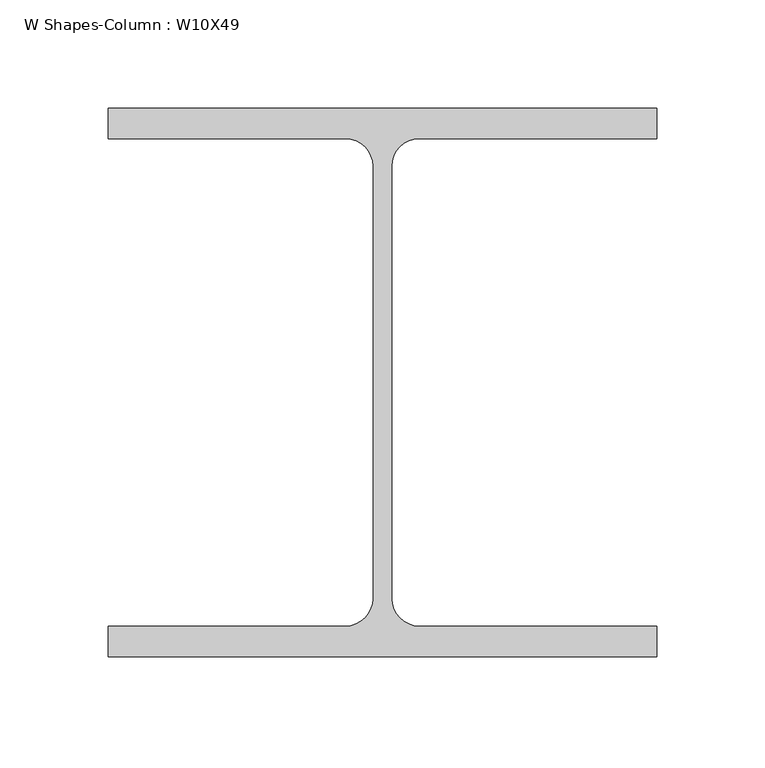
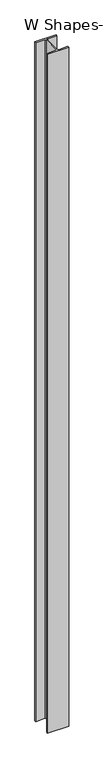
"""IFC4 building model written with IfcOpenShell, lengths in millimetres: column geometry, W Shapes-Column : W10X49."""

from ifc_helpers import new_model, si_unit, point, frame, frame_2d, origin, place, context, project, spatial, polyline, circle_curve, trimmed, segment, composite_curve, outline, extrude, source, transform, mapped, element, save


def w_shapes_column_w10x49_b9b2aca3(model_context):
    return source(origin(), model_context, "Body", "SweptSolid", [
        extrude(outline(composite_curve([segment(polyline([(127.0, 127.0), (127.0, 112.776), (17.018, 112.776)]), True, "CONTINUOUS"), segment(trimmed(circle_curve(frame_2d((17.018, 100.076)), 12.7), [point((17.018, 112.776))], [point((4.318, 100.076))], True, "CARTESIAN"), True, "CONTINUOUS"), segment(polyline([(4.318, 100.076), (4.318, -100.076)]), True, "CONTINUOUS"), segment(trimmed(circle_curve(frame_2d((17.018, -100.076)), 12.7), [point((4.318, -100.076))], [point((17.018, -112.776))], True, "CARTESIAN"), True, "CONTINUOUS"), segment(polyline([(17.018, -112.776), (127.0, -112.776), (127.0, -127.0), (-127.0, -127.0), (-127.0, -112.776), (-17.018, -112.776)]), True, "CONTINUOUS"), segment(trimmed(circle_curve(frame_2d((-17.018, -100.076)), 12.7), [point((-17.018, -112.776))], [point((-4.318, -100.076))], True, "CARTESIAN"), True, "CONTINUOUS"), segment(polyline([(-4.318, -100.076), (-4.318, 100.076)]), True, "CONTINUOUS"), segment(trimmed(circle_curve(frame_2d((-17.018, 100.076)), 12.7), [point((-4.318, 100.076))], [point((-17.018, 112.776))], True, "CARTESIAN"), True, "CONTINUOUS"), segment(polyline([(-17.018, 112.776), (-127.0, 112.776), (-127.0, 127.0), (127.0, 127.0)]), True, "CONTINUOUS")], self_intersect=False)), frame((0.0, 0.0, 2133.9), z_axis=(0.0, 0.0, 1.0), x_axis=(1.0, 0.0, 0.0)), (0.0, 0.0, 1.0), 8534.0),
    ])


if __name__ == "__main__":
    model = new_model("IFC4")
    model_context = context("Model", 3, world=origin())
    ifc_project = project(units=[si_unit("LENGTHUNIT", "METRE", prefix="MILLI")], contexts=[model_context])
    site = spatial("IfcSite", under=ifc_project)
    building = spatial("IfcBuilding", under=site)
    placement = place(None, origin())
    w_shapes_column_w10x49_shape = w_shapes_column_w10x49_b9b2aca3(model_context)
    element("IfcColumn", 1, ObjectType="W Shapes-Column : W10X49", at=placement, inside=building, context=model_context, shape_type="MappedRepresentation", body=[
        mapped(w_shapes_column_w10x49_shape, transform((0.0, 0.0, 0.0), x_axis=(1.0, 0.0, 0.0), y_axis=(0.0, 1.0, 0.0), z_axis=(0.0, 0.0, 1.0))),
    ])
    save(model, "model.ifc")

# Revit data of these elements
# Type "W Shapes-Column : W10X49"
#   Section Name Key = "W10X49"
#   Width = 10.000"
#   Web Thickness = 0.340"
#   Web Fillet = 0.500"
#   Warping Constant = 2070.00 in⁶
#   Torsional Moment of Inertia = 1.39 in⁴
#   Section Area = 14.40 in²
#   Plastic Modulus weak axis = 28.30 in³
#   Plastic Modulus strong axis = 60.40 in³
#   Perimeter = 4.875 ft²/ft
#   Nominal Weight = 49.00 lbf/ft
#   Moment of Inertia weak axis = 93.40 in⁴
#   Moment of Inertia strong axis = 272.00 in⁴
#   Height = 10.000"
#   Flange Thickness = 0.560"
#   Elastic Modulus weak axis = 18.70 in³
#   Elastic Modulus strong axis = 54.60 in³
#   Clear Web Height = 0' - 7 1/2"
#   Centroid Vertical = 5.000"
#   Centroid Horizontal = 5.000"
#   Bolt Spacing = 0' - 5 1/2"
#   Structural Material [instance default] = Steel ASTM A992
#   Principal Axes Angle = 0
# Element 1 (IfcColumn, "W Shapes-Column : W10X49")
#   Materials on its faces: "Steel ASTM A992"
# Materials
#   "Steel ASTM A992": class "Metal", colour RGB 199 199 199, transparency 0, Description = "Structural steel 50ksi", Cost = 0
